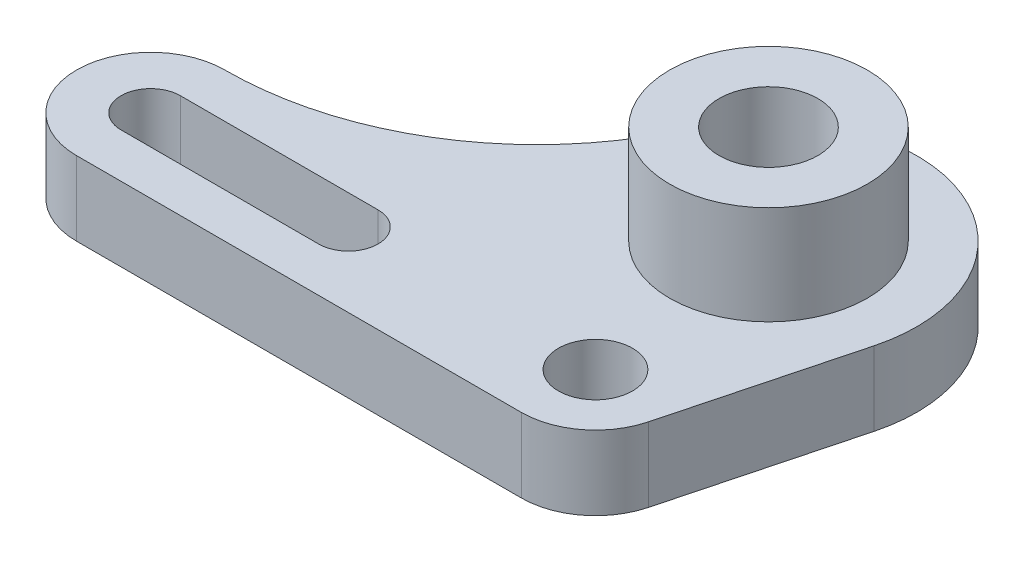
ISO-10303-21;
HEADER;
FILE_DESCRIPTION(('STEP AP214'),'2;1');
FILE_NAME('part.step','',(''),(''),'','','');
FILE_SCHEMA(('AUTOMOTIVE_DESIGN { 1 0 10303 214 1 1 1 1 }'));
ENDSEC;
DATA;
#1=APPLICATION_CONTEXT('core data for automotive mechanical design processes');
#2=APPLICATION_PROTOCOL_DEFINITION('international standard','automotive_design',2000,#1);
#3=PRODUCT_CONTEXT('',#1,'mechanical');
#4=PRODUCT('Part','Part','',(#3));
#5=PRODUCT_RELATED_PRODUCT_CATEGORY('part','',(#4));
#6=PRODUCT_DEFINITION_FORMATION('','',#4);
#7=PRODUCT_DEFINITION_CONTEXT('part definition',#1,'design');
#8=PRODUCT_DEFINITION('design','',#6,#7);
#9=PRODUCT_DEFINITION_SHAPE('','',#8);
#10=(LENGTH_UNIT() NAMED_UNIT(*) SI_UNIT(.MILLI.,.METRE.));
#11=(NAMED_UNIT(*) PLANE_ANGLE_UNIT() SI_UNIT($,.RADIAN.));
#12=(NAMED_UNIT(*) SI_UNIT($,.STERADIAN.) SOLID_ANGLE_UNIT());
#13=UNCERTAINTY_MEASURE_WITH_UNIT(LENGTH_MEASURE(1.E-05),#10,'distance_accuracy_value','');
#14=(GEOMETRIC_REPRESENTATION_CONTEXT(3) GLOBAL_UNCERTAINTY_ASSIGNED_CONTEXT((#13)) GLOBAL_UNIT_ASSIGNED_CONTEXT((#10,
#11,#12)) REPRESENTATION_CONTEXT('',''));
#15=CARTESIAN_POINT('',(0.,0.,0.));
#16=DIRECTION('',(0.,0.,1.));
#17=DIRECTION('',(1.,0.,0.));
#18=AXIS2_PLACEMENT_3D('',#15,#16,#17);
#19=CARTESIAN_POINT('',(0.,15.,0.));
#20=DIRECTION('',(0.,-1.,0.));
#21=DIRECTION('',(0.,0.,-1.));
#22=AXIS2_PLACEMENT_3D('',#19,#20,#21);
#23=CYLINDRICAL_SURFACE('',#22,15.);
#24=CARTESIAN_POINT('',(0.,0.,0.));
#25=DIRECTION('',(0.,1.,0.));
#26=DIRECTION('',(0.,0.,1.));
#27=AXIS2_PLACEMENT_3D('',#24,#25,#26);
#28=CIRCLE('',#27,15.);
#29=CARTESIAN_POINT('',(0.,0.,-15.));
#30=VERTEX_POINT('',#29);
#31=CARTESIAN_POINT('',(0.,0.,15.));
#32=VERTEX_POINT('',#31);
#33=EDGE_CURVE('E153',#30,#32,#28,.T.);
#34=ORIENTED_EDGE('',*,*,#33,.T.);
#35=DIRECTION('',(0.,-1.,0.));
#36=VECTOR('',#35,1.);
#37=CARTESIAN_POINT('',(0.,15.,15.));
#38=LINE('',#37,#36);
#39=CARTESIAN_POINT('',(0.,15.,15.));
#40=VERTEX_POINT('',#39);
#41=EDGE_CURVE('E45',#40,#32,#38,.T.);
#42=ORIENTED_EDGE('',*,*,#41,.F.);
#43=CARTESIAN_POINT('',(0.,15.,0.));
#44=DIRECTION('',(0.,1.,0.));
#45=DIRECTION('',(0.,0.,1.));
#46=AXIS2_PLACEMENT_3D('',#43,#44,#45);
#47=CIRCLE('',#46,15.);
#48=CARTESIAN_POINT('',(0.,15.,-15.));
#49=VERTEX_POINT('',#48);
#50=EDGE_CURVE('E160',#49,#40,#47,.T.);
#51=ORIENTED_EDGE('',*,*,#50,.F.);
#52=DIRECTION('',(0.,-1.,0.));
#53=VECTOR('',#52,1.);
#54=CARTESIAN_POINT('',(0.,15.,-15.));
#55=LINE('',#54,#53);
#56=EDGE_CURVE('E174',#49,#30,#55,.T.);
#57=ORIENTED_EDGE('',*,*,#56,.T.);
#58=EDGE_LOOP('',(#34,#42,#51,#57));
#59=FACE_BOUND('',#58,.T.);
#60=ADVANCED_FACE('F39',(#59),#23,.T.);
#61=CARTESIAN_POINT('',(0.,15.,15.));
#62=DIRECTION('',(0.,0.,-1.));
#63=DIRECTION('',(-1.,0.,0.));
#64=AXIS2_PLACEMENT_3D('',#61,#62,#63);
#65=PLANE('',#64);
#66=DIRECTION('',(1.,0.,0.));
#67=VECTOR('',#66,1.);
#68=CARTESIAN_POINT('',(0.,0.,15.));
#69=LINE('',#68,#67);
#70=CARTESIAN_POINT('',(90.,0.,15.));
#71=VERTEX_POINT('',#70);
#72=EDGE_CURVE('E173',#32,#71,#69,.T.);
#73=ORIENTED_EDGE('',*,*,#72,.T.);
#74=DIRECTION('',(0.,-1.,0.));
#75=VECTOR('',#74,1.);
#76=CARTESIAN_POINT('',(90.,15.,15.));
#77=LINE('',#76,#75);
#78=CARTESIAN_POINT('',(90.,15.,15.));
#79=VERTEX_POINT('',#78);
#80=EDGE_CURVE('E191',#79,#71,#77,.T.);
#81=ORIENTED_EDGE('',*,*,#80,.F.);
#82=DIRECTION('',(1.,0.,0.));
#83=VECTOR('',#82,1.);
#84=CARTESIAN_POINT('',(0.,15.,15.));
#85=LINE('',#84,#83);
#86=EDGE_CURVE('E159',#40,#79,#85,.T.);
#87=ORIENTED_EDGE('',*,*,#86,.F.);
#88=ORIENTED_EDGE('',*,*,#41,.T.);
#89=EDGE_LOOP('',(#73,#81,#87,#88));
#90=FACE_BOUND('',#89,.T.);
#91=ADVANCED_FACE('F205',(#90),#65,.F.);
#92=CARTESIAN_POINT('',(90.,15.,0.));
#93=DIRECTION('',(0.,-1.,0.));
#94=DIRECTION('',(0.,0.,-1.));
#95=AXIS2_PLACEMENT_3D('',#92,#93,#94);
#96=CYLINDRICAL_SURFACE('',#95,15.);
#97=CARTESIAN_POINT('',(90.,0.,0.));
#98=DIRECTION('',(0.,1.,0.));
#99=DIRECTION('',(0.,0.,1.));
#100=AXIS2_PLACEMENT_3D('',#97,#98,#99);
#101=CIRCLE('',#100,15.);
#102=CARTESIAN_POINT('',(104.507658043473,0.,3.81154274456587));
#103=VERTEX_POINT('',#102);
#104=EDGE_CURVE('E178',#71,#103,#101,.T.);
#105=ORIENTED_EDGE('',*,*,#104,.T.);
#106=DIRECTION('',(0.,-1.,0.));
#107=VECTOR('',#106,1.);
#108=CARTESIAN_POINT('',(104.507658043473,15.,3.81154274456587));
#109=LINE('',#108,#107);
#110=CARTESIAN_POINT('',(104.507658043473,15.,3.81154274456587));
#111=VERTEX_POINT('',#110);
#112=EDGE_CURVE('E193',#111,#103,#109,.T.);
#113=ORIENTED_EDGE('',*,*,#112,.F.);
#114=CARTESIAN_POINT('',(90.,15.,0.));
#115=DIRECTION('',(0.,1.,0.));
#116=DIRECTION('',(0.,0.,1.));
#117=AXIS2_PLACEMENT_3D('',#114,#115,#116);
#118=CIRCLE('',#117,15.);
#119=EDGE_CURVE('E162',#79,#111,#118,.T.);
#120=ORIENTED_EDGE('',*,*,#119,.F.);
#121=ORIENTED_EDGE('',*,*,#80,.T.);
#122=EDGE_LOOP('',(#105,#113,#120,#121));
#123=FACE_BOUND('',#122,.T.);
#124=ADVANCED_FACE('F211',(#123),#96,.T.);
#125=CARTESIAN_POINT('',(114.015316086946,15.,-32.3769145108683));
#126=DIRECTION('',(-0.967177202898201,0.,-0.254102849637725));
#127=DIRECTION('',(-0.254102849637725,0.,0.967177202898201));
#128=AXIS2_PLACEMENT_3D('',#125,#126,#127);
#129=PLANE('',#128);
#130=DIRECTION('',(0.254102849637725,0.,-0.967177202898201));
#131=VECTOR('',#130,1.);
#132=CARTESIAN_POINT('',(114.015316086946,0.,-32.3769145108683));
#133=LINE('',#132,#131);
#134=CARTESIAN_POINT('',(114.015316086946,0.,-32.3769145108683));
#135=VERTEX_POINT('',#134);
#136=EDGE_CURVE('E176',#103,#135,#133,.T.);
#137=ORIENTED_EDGE('',*,*,#136,.T.);
#138=DIRECTION('',(0.,-1.,0.));
#139=VECTOR('',#138,1.);
#140=CARTESIAN_POINT('',(114.015316086946,15.,-32.3769145108683));
#141=LINE('',#140,#139);
#142=CARTESIAN_POINT('',(114.015316086946,15.,-32.3769145108683));
#143=VERTEX_POINT('',#142);
#144=EDGE_CURVE('E190',#143,#135,#141,.T.);
#145=ORIENTED_EDGE('',*,*,#144,.F.);
#146=DIRECTION('',(0.254102849637725,0.,-0.967177202898201));
#147=VECTOR('',#146,1.);
#148=CARTESIAN_POINT('',(114.015316086946,15.,-32.3769145108683));
#149=LINE('',#148,#147);
#150=EDGE_CURVE('E164',#111,#143,#149,.T.);
#151=ORIENTED_EDGE('',*,*,#150,.F.);
#152=ORIENTED_EDGE('',*,*,#112,.T.);
#153=EDGE_LOOP('',(#137,#145,#151,#152));
#154=FACE_BOUND('',#153,.T.);
#155=ADVANCED_FACE('F212',(#154),#129,.F.);
#156=CARTESIAN_POINT('',(85.,15.,-40.));
#157=DIRECTION('',(0.,-1.,0.));
#158=DIRECTION('',(0.,0.,-1.));
#159=AXIS2_PLACEMENT_3D('',#156,#157,#158);
#160=CYLINDRICAL_SURFACE('',#159,30.);
#161=CARTESIAN_POINT('',(85.,0.,-40.));
#162=DIRECTION('',(0.,1.,0.));
#163=DIRECTION('',(0.,0.,1.));
#164=AXIS2_PLACEMENT_3D('',#161,#162,#163);
#165=CIRCLE('',#164,30.);
#166=CARTESIAN_POINT('',(57.6341463414634,0.,-52.2926829268293));
#167=VERTEX_POINT('',#166);
#168=EDGE_CURVE('E177',#135,#167,#165,.T.);
#169=ORIENTED_EDGE('',*,*,#168,.T.);
#170=DIRECTION('',(0.,-1.,0.));
#171=VECTOR('',#170,1.);
#172=CARTESIAN_POINT('',(57.6341463414634,15.,-52.2926829268293));
#173=LINE('',#172,#171);
#174=CARTESIAN_POINT('',(57.6341463414634,15.,-52.2926829268293));
#175=VERTEX_POINT('',#174);
#176=EDGE_CURVE('E183',#175,#167,#173,.T.);
#177=ORIENTED_EDGE('',*,*,#176,.F.);
#178=CARTESIAN_POINT('',(85.,15.,-40.));
#179=DIRECTION('',(0.,1.,0.));
#180=DIRECTION('',(0.,0.,1.));
#181=AXIS2_PLACEMENT_3D('',#178,#179,#180);
#182=CIRCLE('',#181,30.);
#183=EDGE_CURVE('E170',#143,#175,#182,.T.);
#184=ORIENTED_EDGE('',*,*,#183,.F.);
#185=ORIENTED_EDGE('',*,*,#144,.T.);
#186=EDGE_LOOP('',(#169,#177,#184,#185));
#187=FACE_BOUND('',#186,.T.);
#188=ADVANCED_FACE('F221',(#187),#160,.T.);
#189=CARTESIAN_POINT('',(-1.14491749414469E-13,15.,-78.1818181818183));
#190=DIRECTION('',(0.,-1.,0.));
#191=DIRECTION('',(0.,0.,-1.));
#192=AXIS2_PLACEMENT_3D('',#189,#190,#191);
#193=CYLINDRICAL_SURFACE('',#192,63.1818181818183);
#194=CARTESIAN_POINT('',(-1.14491749414469E-13,0.,-78.1818181818183));
#195=DIRECTION('',(0.,-1.,0.));
#196=DIRECTION('',(0.,0.,1.));
#197=AXIS2_PLACEMENT_3D('',#194,#195,#196);
#198=CIRCLE('',#197,63.1818181818183);
#199=EDGE_CURVE('E161',#167,#30,#198,.T.);
#200=ORIENTED_EDGE('',*,*,#199,.T.);
#201=ORIENTED_EDGE('',*,*,#56,.F.);
#202=CARTESIAN_POINT('',(-1.14491749414469E-13,15.,-78.1818181818183));
#203=DIRECTION('',(0.,-1.,0.));
#204=DIRECTION('',(0.,0.,1.));
#205=AXIS2_PLACEMENT_3D('',#202,#203,#204);
#206=CIRCLE('',#205,63.1818181818183);
#207=EDGE_CURVE('E166',#175,#49,#206,.T.);
#208=ORIENTED_EDGE('',*,*,#207,.F.);
#209=ORIENTED_EDGE('',*,*,#176,.T.);
#210=EDGE_LOOP('',(#200,#201,#208,#209));
#211=FACE_BOUND('',#210,.T.);
#212=ADVANCED_FACE('F225',(#211),#193,.F.);
#213=CARTESIAN_POINT('',(0.,15.,0.));
#214=DIRECTION('',(0.,1.,0.));
#215=DIRECTION('',(0.,0.,1.));
#216=AXIS2_PLACEMENT_3D('',#213,#214,#215);
#217=PLANE('',#216);
#218=CARTESIAN_POINT('',(85.,15.,-40.));
#219=DIRECTION('',(0.,1.,0.));
#220=DIRECTION('',(0.,0.,1.));
#221=AXIS2_PLACEMENT_3D('',#218,#219,#220);
#222=CIRCLE('',#221,20.);
#223=CARTESIAN_POINT('',(85.,15.,-20.));
#224=VERTEX_POINT('',#223);
#225=EDGE_CURVE('E11',#224,#224,#222,.T.);
#226=ORIENTED_EDGE('',*,*,#225,.F.);
#227=EDGE_LOOP('',(#226));
#228=FACE_BOUND('',#227,.T.);
#229=CARTESIAN_POINT('',(90.,15.,0.));
#230=DIRECTION('',(0.,1.,0.));
#231=DIRECTION('',(0.,0.,1.));
#232=AXIS2_PLACEMENT_3D('',#229,#230,#231);
#233=CIRCLE('',#232,7.50000000000001);
#234=CARTESIAN_POINT('',(90.,15.,7.50000000000001));
#235=VERTEX_POINT('',#234);
#236=EDGE_CURVE('E137',#235,#235,#233,.T.);
#237=ORIENTED_EDGE('',*,*,#236,.F.);
#238=EDGE_LOOP('',(#237));
#239=FACE_BOUND('',#238,.T.);
#240=CARTESIAN_POINT('',(0.,15.,0.));
#241=DIRECTION('',(0.,1.,0.));
#242=DIRECTION('',(0.,0.,1.));
#243=AXIS2_PLACEMENT_3D('',#240,#241,#242);
#244=CIRCLE('',#243,6.);
#245=CARTESIAN_POINT('',(0.,15.,-6.));
#246=VERTEX_POINT('',#245);
#247=CARTESIAN_POINT('',(0.,15.,6.));
#248=VERTEX_POINT('',#247);
#249=EDGE_CURVE('E53',#246,#248,#244,.T.);
#250=ORIENTED_EDGE('',*,*,#249,.F.);
#251=DIRECTION('',(-1.,0.,0.));
#252=VECTOR('',#251,1.);
#253=CARTESIAN_POINT('',(0.,15.,-6.));
#254=LINE('',#253,#252);
#255=CARTESIAN_POINT('',(40.,15.,-6.));
#256=VERTEX_POINT('',#255);
#257=EDGE_CURVE('E133',#256,#246,#254,.T.);
#258=ORIENTED_EDGE('',*,*,#257,.F.);
#259=CARTESIAN_POINT('',(40.,15.,0.));
#260=DIRECTION('',(0.,1.,0.));
#261=DIRECTION('',(0.,0.,1.));
#262=AXIS2_PLACEMENT_3D('',#259,#260,#261);
#263=CIRCLE('',#262,6.);
#264=CARTESIAN_POINT('',(40.,15.,6.));
#265=VERTEX_POINT('',#264);
#266=EDGE_CURVE('E140',#265,#256,#263,.T.);
#267=ORIENTED_EDGE('',*,*,#266,.F.);
#268=DIRECTION('',(1.,0.,0.));
#269=VECTOR('',#268,1.);
#270=CARTESIAN_POINT('',(0.,15.,6.));
#271=LINE('',#270,#269);
#272=EDGE_CURVE('E148',#248,#265,#271,.T.);
#273=ORIENTED_EDGE('',*,*,#272,.F.);
#274=EDGE_LOOP('',(#250,#258,#267,#273));
#275=FACE_BOUND('',#274,.T.);
#276=ORIENTED_EDGE('',*,*,#50,.T.);
#277=ORIENTED_EDGE('',*,*,#86,.T.);
#278=ORIENTED_EDGE('',*,*,#119,.T.);
#279=ORIENTED_EDGE('',*,*,#150,.T.);
#280=ORIENTED_EDGE('',*,*,#183,.T.);
#281=ORIENTED_EDGE('',*,*,#207,.T.);
#282=EDGE_LOOP('',(#276,#277,#278,#279,#280,#281));
#283=FACE_BOUND('',#282,.T.);
#284=ADVANCED_FACE('F217',(#228,#239,#275,#283),#217,.T.);
#285=CARTESIAN_POINT('',(0.,0.,0.));
#286=DIRECTION('',(0.,1.,0.));
#287=DIRECTION('',(0.,0.,1.));
#288=AXIS2_PLACEMENT_3D('',#285,#286,#287);
#289=PLANE('',#288);
#290=CARTESIAN_POINT('',(90.,0.,0.));
#291=DIRECTION('',(0.,1.,0.));
#292=DIRECTION('',(0.,0.,1.));
#293=AXIS2_PLACEMENT_3D('',#290,#291,#292);
#294=CIRCLE('',#293,7.50000000000001);
#295=CARTESIAN_POINT('',(90.,0.,7.50000000000001));
#296=VERTEX_POINT('',#295);
#297=EDGE_CURVE('E150',#296,#296,#294,.T.);
#298=ORIENTED_EDGE('',*,*,#297,.T.);
#299=EDGE_LOOP('',(#298));
#300=FACE_BOUND('',#299,.T.);
#301=DIRECTION('',(-1.,0.,0.));
#302=VECTOR('',#301,1.);
#303=CARTESIAN_POINT('',(0.,0.,-6.));
#304=LINE('',#303,#302);
#305=CARTESIAN_POINT('',(40.,0.,-6.));
#306=VERTEX_POINT('',#305);
#307=CARTESIAN_POINT('',(0.,0.,-6.));
#308=VERTEX_POINT('',#307);
#309=EDGE_CURVE('E124',#306,#308,#304,.T.);
#310=ORIENTED_EDGE('',*,*,#309,.T.);
#311=CARTESIAN_POINT('',(0.,0.,0.));
#312=DIRECTION('',(0.,1.,0.));
#313=DIRECTION('',(0.,0.,1.));
#314=AXIS2_PLACEMENT_3D('',#311,#312,#313);
#315=CIRCLE('',#314,6.);
#316=CARTESIAN_POINT('',(0.,0.,6.));
#317=VERTEX_POINT('',#316);
#318=EDGE_CURVE('E120',#308,#317,#315,.T.);
#319=ORIENTED_EDGE('',*,*,#318,.T.);
#320=DIRECTION('',(1.,0.,0.));
#321=VECTOR('',#320,1.);
#322=CARTESIAN_POINT('',(0.,0.,6.));
#323=LINE('',#322,#321);
#324=CARTESIAN_POINT('',(40.,0.,6.));
#325=VERTEX_POINT('',#324);
#326=EDGE_CURVE('E130',#317,#325,#323,.T.);
#327=ORIENTED_EDGE('',*,*,#326,.T.);
#328=CARTESIAN_POINT('',(40.,0.,0.));
#329=DIRECTION('',(0.,1.,0.));
#330=DIRECTION('',(0.,0.,1.));
#331=AXIS2_PLACEMENT_3D('',#328,#329,#330);
#332=CIRCLE('',#331,6.);
#333=EDGE_CURVE('E61',#325,#306,#332,.T.);
#334=ORIENTED_EDGE('',*,*,#333,.T.);
#335=EDGE_LOOP('',(#310,#319,#327,#334));
#336=FACE_BOUND('',#335,.T.);
#337=ORIENTED_EDGE('',*,*,#33,.F.);
#338=ORIENTED_EDGE('',*,*,#199,.F.);
#339=ORIENTED_EDGE('',*,*,#168,.F.);
#340=ORIENTED_EDGE('',*,*,#136,.F.);
#341=ORIENTED_EDGE('',*,*,#104,.F.);
#342=ORIENTED_EDGE('',*,*,#72,.F.);
#343=EDGE_LOOP('',(#337,#338,#339,#340,#341,#342));
#344=FACE_BOUND('',#343,.T.);
#345=ADVANCED_FACE('F134',(#300,#336,#344),#289,.F.);
#346=CARTESIAN_POINT('',(0.,0.,0.));
#347=DIRECTION('',(0.,1.,0.));
#348=DIRECTION('',(0.,0.,1.));
#349=AXIS2_PLACEMENT_3D('',#346,#347,#348);
#350=CYLINDRICAL_SURFACE('',#349,6.);
#351=ORIENTED_EDGE('',*,*,#249,.T.);
#352=DIRECTION('',(0.,1.,0.));
#353=VECTOR('',#352,1.);
#354=CARTESIAN_POINT('',(0.,0.,6.));
#355=LINE('',#354,#353);
#356=EDGE_CURVE('E111',#317,#248,#355,.T.);
#357=ORIENTED_EDGE('',*,*,#356,.F.);
#358=ORIENTED_EDGE('',*,*,#318,.F.);
#359=DIRECTION('',(0.,1.,0.));
#360=VECTOR('',#359,1.);
#361=CARTESIAN_POINT('',(0.,0.,-6.));
#362=LINE('',#361,#360);
#363=EDGE_CURVE('E151',#308,#246,#362,.T.);
#364=ORIENTED_EDGE('',*,*,#363,.T.);
#365=EDGE_LOOP('',(#351,#357,#358,#364));
#366=FACE_BOUND('',#365,.T.);
#367=ADVANCED_FACE('F119',(#366),#350,.F.);
#368=CARTESIAN_POINT('',(0.,0.,-6.));
#369=DIRECTION('',(0.,0.,-1.));
#370=DIRECTION('',(-1.,0.,0.));
#371=AXIS2_PLACEMENT_3D('',#368,#369,#370);
#372=PLANE('',#371);
#373=ORIENTED_EDGE('',*,*,#257,.T.);
#374=ORIENTED_EDGE('',*,*,#363,.F.);
#375=ORIENTED_EDGE('',*,*,#309,.F.);
#376=DIRECTION('',(0.,1.,0.));
#377=VECTOR('',#376,1.);
#378=CARTESIAN_POINT('',(40.,0.,-6.));
#379=LINE('',#378,#377);
#380=EDGE_CURVE('E152',#306,#256,#379,.T.);
#381=ORIENTED_EDGE('',*,*,#380,.T.);
#382=EDGE_LOOP('',(#373,#374,#375,#381));
#383=FACE_BOUND('',#382,.T.);
#384=ADVANCED_FACE('F287',(#383),#372,.F.);
#385=CARTESIAN_POINT('',(40.,0.,0.));
#386=DIRECTION('',(0.,1.,0.));
#387=DIRECTION('',(0.,0.,1.));
#388=AXIS2_PLACEMENT_3D('',#385,#386,#387);
#389=CYLINDRICAL_SURFACE('',#388,6.);
#390=ORIENTED_EDGE('',*,*,#266,.T.);
#391=ORIENTED_EDGE('',*,*,#380,.F.);
#392=ORIENTED_EDGE('',*,*,#333,.F.);
#393=DIRECTION('',(0.,1.,0.));
#394=VECTOR('',#393,1.);
#395=CARTESIAN_POINT('',(40.,0.,6.));
#396=LINE('',#395,#394);
#397=EDGE_CURVE('E121',#325,#265,#396,.T.);
#398=ORIENTED_EDGE('',*,*,#397,.T.);
#399=EDGE_LOOP('',(#390,#391,#392,#398));
#400=FACE_BOUND('',#399,.T.);
#401=ADVANCED_FACE('F298',(#400),#389,.F.);
#402=CARTESIAN_POINT('',(0.,0.,6.));
#403=DIRECTION('',(0.,0.,1.));
#404=DIRECTION('',(1.,0.,0.));
#405=AXIS2_PLACEMENT_3D('',#402,#403,#404);
#406=PLANE('',#405);
#407=ORIENTED_EDGE('',*,*,#272,.T.);
#408=ORIENTED_EDGE('',*,*,#397,.F.);
#409=ORIENTED_EDGE('',*,*,#326,.F.);
#410=ORIENTED_EDGE('',*,*,#356,.T.);
#411=EDGE_LOOP('',(#407,#408,#409,#410));
#412=FACE_BOUND('',#411,.T.);
#413=ADVANCED_FACE('F126',(#412),#406,.F.);
#414=CARTESIAN_POINT('',(90.,0.,0.));
#415=DIRECTION('',(0.,1.,0.));
#416=DIRECTION('',(0.,0.,1.));
#417=AXIS2_PLACEMENT_3D('',#414,#415,#416);
#418=CYLINDRICAL_SURFACE('',#417,7.50000000000001);
#419=ORIENTED_EDGE('',*,*,#297,.F.);
#420=EDGE_LOOP('',(#419));
#421=FACE_BOUND('',#420,.T.);
#422=ORIENTED_EDGE('',*,*,#236,.T.);
#423=EDGE_LOOP('',(#422));
#424=FACE_BOUND('',#423,.T.);
#425=ADVANCED_FACE('F316',(#421,#424),#418,.F.);
#426=CARTESIAN_POINT('',(85.,35.,-40.));
#427=DIRECTION('',(0.,1.,0.));
#428=DIRECTION('',(0.,0.,1.));
#429=AXIS2_PLACEMENT_3D('',#426,#427,#428);
#430=PLANE('',#429);
#431=CARTESIAN_POINT('',(85.,35.,-40.));
#432=DIRECTION('',(0.,1.,0.));
#433=DIRECTION('',(0.,0.,1.));
#434=AXIS2_PLACEMENT_3D('',#431,#432,#433);
#435=CIRCLE('',#434,20.);
#436=CARTESIAN_POINT('',(85.,35.,-20.));
#437=VERTEX_POINT('',#436);
#438=EDGE_CURVE('E375',#437,#437,#435,.T.);
#439=ORIENTED_EDGE('',*,*,#438,.T.);
#440=EDGE_LOOP('',(#439));
#441=FACE_BOUND('',#440,.T.);
#442=CARTESIAN_POINT('',(85.,35.,-40.));
#443=DIRECTION('',(0.,1.,0.));
#444=DIRECTION('',(0.,0.,1.));
#445=AXIS2_PLACEMENT_3D('',#442,#443,#444);
#446=CIRCLE('',#445,9.99999999999999);
#447=CARTESIAN_POINT('',(85.,35.,-30.));
#448=VERTEX_POINT('',#447);
#449=EDGE_CURVE('E370',#448,#448,#446,.T.);
#450=ORIENTED_EDGE('',*,*,#449,.F.);
#451=EDGE_LOOP('',(#450));
#452=FACE_BOUND('',#451,.T.);
#453=ADVANCED_FACE('F322',(#441,#452),#430,.T.);
#454=CARTESIAN_POINT('',(85.,35.,-40.));
#455=DIRECTION('',(0.,-1.,0.));
#456=DIRECTION('',(0.,0.,-1.));
#457=AXIS2_PLACEMENT_3D('',#454,#455,#456);
#458=CYLINDRICAL_SURFACE('',#457,20.);
#459=ORIENTED_EDGE('',*,*,#438,.F.);
#460=EDGE_LOOP('',(#459));
#461=FACE_BOUND('',#460,.T.);
#462=ORIENTED_EDGE('',*,*,#225,.T.);
#463=EDGE_LOOP('',(#462));
#464=FACE_BOUND('',#463,.T.);
#465=ADVANCED_FACE('F343',(#461,#464),#458,.T.);
#466=CARTESIAN_POINT('',(85.,35.,-40.));
#467=DIRECTION('',(0.,-1.,0.));
#468=DIRECTION('',(0.,0.,-1.));
#469=AXIS2_PLACEMENT_3D('',#466,#467,#468);
#470=CYLINDRICAL_SURFACE('',#469,9.99999999999999);
#471=ORIENTED_EDGE('',*,*,#449,.T.);
#472=EDGE_LOOP('',(#471));
#473=FACE_BOUND('',#472,.T.);
#474=CARTESIAN_POINT('',(85.,15.,-40.));
#475=DIRECTION('',(0.,1.,0.));
#476=DIRECTION('',(0.,0.,1.));
#477=AXIS2_PLACEMENT_3D('',#474,#475,#476);
#478=CIRCLE('',#477,9.99999999999999);
#479=CARTESIAN_POINT('',(85.,15.,-30.));
#480=VERTEX_POINT('',#479);
#481=EDGE_CURVE('E367',#480,#480,#478,.T.);
#482=ORIENTED_EDGE('',*,*,#481,.F.);
#483=EDGE_LOOP('',(#482));
#484=FACE_BOUND('',#483,.T.);
#485=ADVANCED_FACE('F331',(#473,#484),#470,.F.);
#486=ORIENTED_EDGE('',*,*,#481,.T.);
#487=EDGE_LOOP('',(#486));
#488=FACE_BOUND('',#487,.T.);
#489=ADVANCED_FACE('F271',(#488),#217,.T.);
#490=CLOSED_SHELL('',(#60,#91,#124,#155,#188,#212,#284,#345,#367,#384,#401,#413,#425,#453,#465,
#485,#489));
#491=MANIFOLD_SOLID_BREP('B2',#490);
#492=ADVANCED_BREP_SHAPE_REPRESENTATION('',(#18,#491),#14);
#493=SHAPE_DEFINITION_REPRESENTATION(#9,#492);
ENDSEC;
END-ISO-10303-21;
